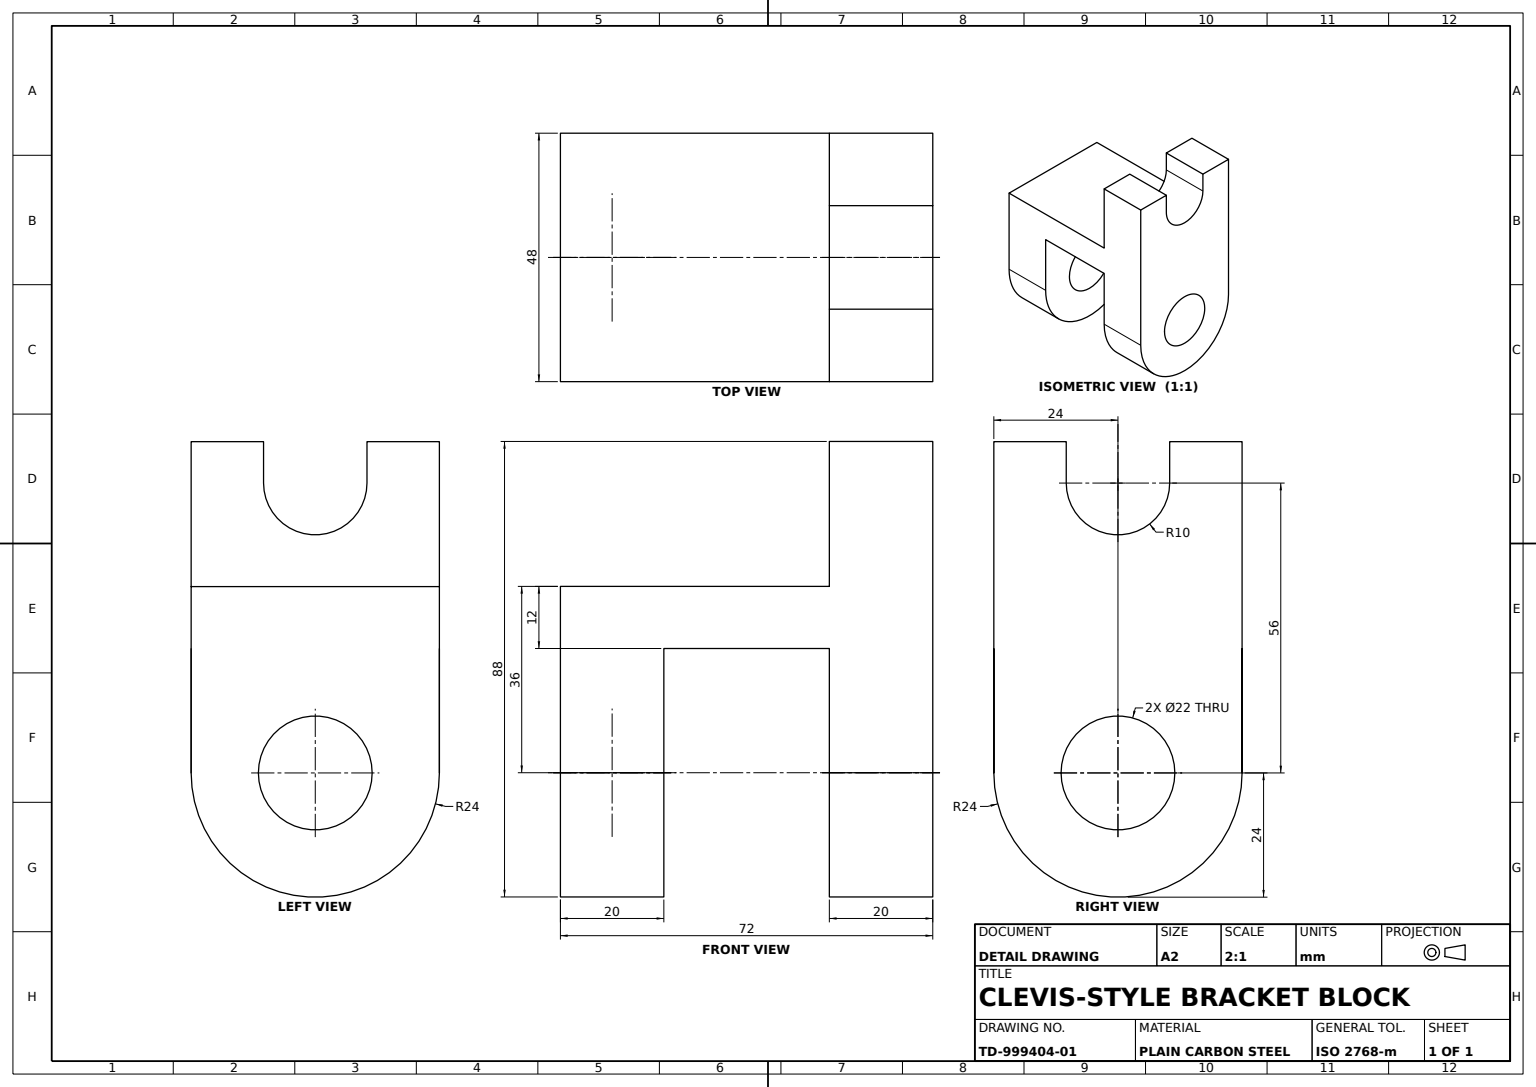
from build123d import *

# Parameters (mm, degrees)
FRONT_LUG_DEPTH            = 20
REAR_LUG_DEPTH             = 20
CONNECTING_BLOCK_PROFILE_W = 48
CONNECTING_BLOCK_PROFILE_H = 32
CONNECTING_BLOCK_DEPTH     = 12
CLEVIS_FORK_DEPTH          = 20
PIN_HOLE_PROFILE_R         = 11
PIN_HOLE_DEPTH             = 99


with BuildPart() as part:
    # Front Lug Profile → Front Lug (new body)
    with BuildSketch(Plane.XY):
        with BuildLine():
            Line((24, 0), (24, 36))
            Line((24, 36), (-24, 36))
            Line((-24, 36), (-24, 0))
            ThreePointArc((-24, 0), (0, -24), (24, 0))
        make_face()
    extrude(amount=-FRONT_LUG_DEPTH)



with BuildPart() as body_2:
    # Rear Lug Profile → Rear Lug (new body)
    with BuildSketch(Plane(origin=(0, 0, -52), x_dir=(-1, 0, 0), z_dir=(0, 0, -1))):
        with BuildLine():
            Line((-24, 0), (-24, 36))
            Line((-24, 36), (24, 36))
            Line((24, 36), (24, 0))
            ThreePointArc((24, 0), (0, -24), (-24, 0))
        make_face()
    extrude(amount=REAR_LUG_DEPTH)


with BuildPart() as part_1:
    add(part.part)

    add(body_2.part)  # Connecting Block merges body 2
    # Connecting Block Profile → Connecting Block (add)
    with BuildSketch(Plane(origin=(0, 36, 0), x_dir=(1, 0, 0), z_dir=(0, 1, 0))):
        with Locations((0, 36)):
            Rectangle(CONNECTING_BLOCK_PROFILE_W, CONNECTING_BLOCK_PROFILE_H)
    extrude(amount=-CONNECTING_BLOCK_DEPTH)

    # Clevis Fork Profile → Clevis Fork (add)
    with BuildSketch(Plane(origin=(0, 0, -72), x_dir=(-1, 0, 0), z_dir=(0, 0, -1))):
        with BuildLine():
            Line((10, 56), (10, 64))
            Line((10, 64), (24, 64))
            Line((24, 64), (24, 36))
            Line((24, 36), (-24, 36))
            Line((-24, 36), (-24, 64))
            Line((-24, 64), (-10, 64))
            Line((-10, 64), (-10, 56))
            ThreePointArc((-10, 56), (0, 46), (10, 56))
        make_face()
    extrude(amount=-CLEVIS_FORK_DEPTH)

    # Pin Hole Profile → Pin Hole (cut)
    with BuildSketch(Plane.XY):
        with Locations(Location((0, 0, 0), (0, 0, 180))):
            Circle(PIN_HOLE_PROFILE_R)
    extrude(amount=-PIN_HOLE_DEPTH, mode=Mode.SUBTRACT)


solid = part_1.part
